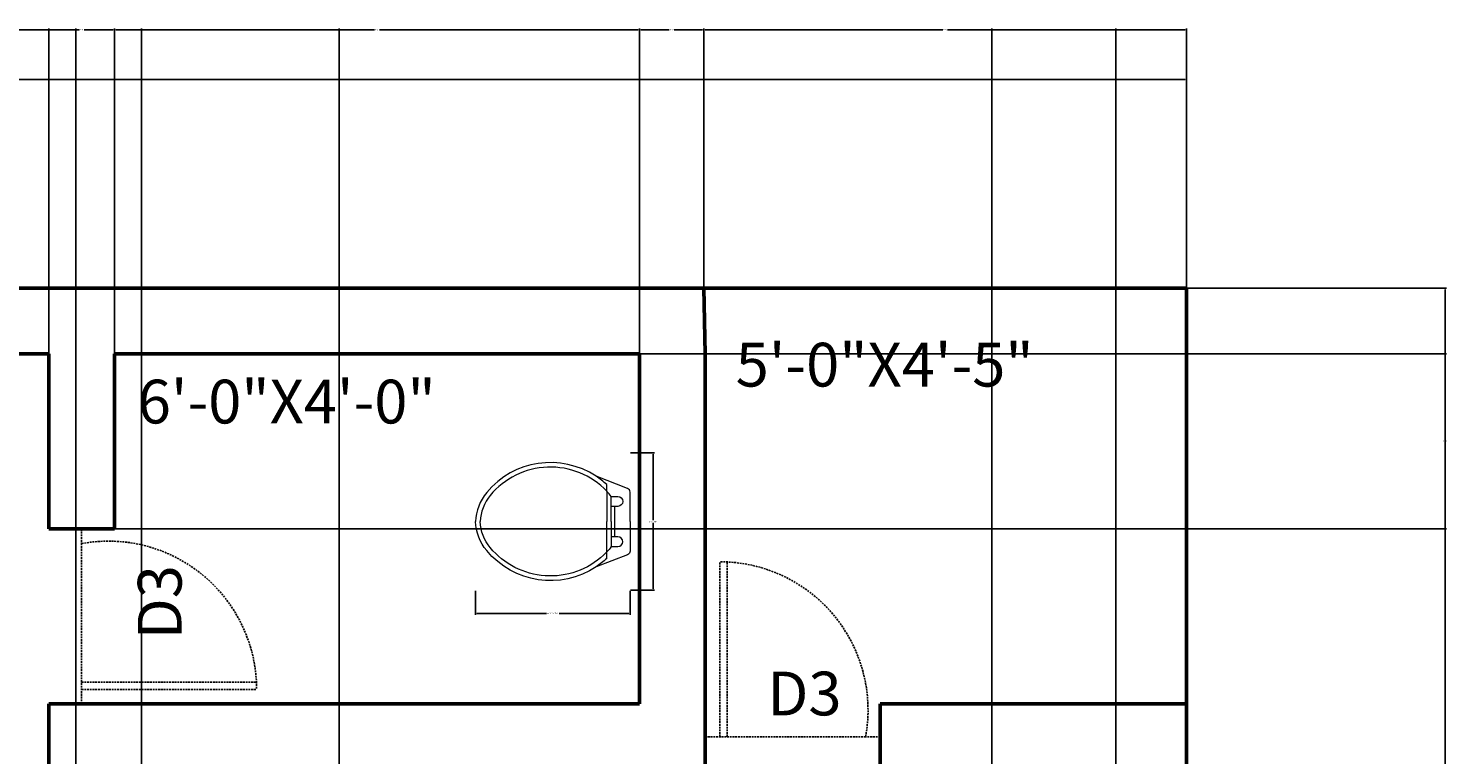
# Model space of a CAD drawing. Units: inches. Extents: x 3 to 576, y -689 to 51.
# Tile 21 of 21: x 381 to 576, y -48 to 51. Entities that reach past the tile are written whole.
import ezdxf

# ---------------------------------------------------------------- set-up
doc = ezdxf.new("R2010")
doc.units = ezdxf.units.IN
doc.header["$MEASUREMENT"] = 0
doc.linetypes.add('DASHED2', pattern=[0.375, 0.25, -0.125])
for name, color, linetype, lineweight in [('A-ANNO-DIMS', 2, 'Continuous', 18), ('A-ANNO-TEXT', 3, 'Continuous', 18), ('A-AREA-IDEN', 7, 'Continuous', 18), ('A-DOOR', 4, 'DASHED2', 25), ('A-FLOR-FIXT', 9, 'Continuous', 18), ('A-WALL', 7, 'Continuous', 50)]:
    doc.layers.add(name, color=color, linetype=linetype, lineweight=lineweight)
doc.styles.get("Standard").update_dxf_attribs({"font": 'arial.ttf'})
doc.dimstyles.get("Standard").update_dxf_attribs({"dimtxt": 0.18, "dimasz": 0.18, "dimexe": 0.18, "dimexo": 0.0625, "dimgap": 0.09, "dimtad": 0, "dimtih": 1, "dimtoh": 1, "dimdec": 0, "dimzin": 0, "dimdsep": 46, "dimlunit": 3, "dimtxsty": 'Standard', "dimcen": 0.09, "dimadec": 0, "dimazin": 0, "dimtfac": 1, "dimtdec": 0, "dimtofl": 0, "dimtmove": 0, "dimatfit": 3, "dimfxl": 1, "dimtolj": 1, "dimtzin": 0, "dimarcsym": 0})

# ---------------------------------------------------------------- blocks, each defined once
blk = doc.blocks.new('*D1')
at = {"layer": 'A-ANNO-DIMS', "color": 0, "lineweight": -2, "transparency": 16777216}
for p, q in [((38.29, 15.75), (38.29, 44.49)), ((38.47, 44.31), (276.45, 44.31)), ((540.11, 44.31), (302.14, 44.31)), ((540.29, 15.75), (540.29, 44.49))]:
    blk.add_line(p, q, dxfattribs=at)
at = {"layer": 'A-ANNO-DIMS', "color": 0, "transparency": 16777216}
for points in [[(38.47, 44.34), (38.47, 44.28), (38.29, 44.31)], [(540.11, 44.34), (540.11, 44.28), (540.29, 44.31)]]:
    blk.add_solid(points, dxfattribs=at)
at = {"layer": 'Defpoints', "color": 0, "transparency": 16777216}
for p in [(540.29, 44.31), (38.29, 15.69), (540.29, 15.69)]:
    blk.add_point(p, dxfattribs=at)
at = {"layer": 'A-ANNO-DIMS', "color": 0, "transparency": 16777216, "insert": (289.29, 44.31), "char_height": 6, "attachment_point": 5}
blk.add_mtext('\\A1;41\'-10"', dxfattribs=at)
blk = doc.blocks.new('WC-2')
for p, q in [((17.99, 12.27), (17.99, 13.16)), ((17.99, 12.27), (17.99, 8.1)), ((17.99, 3.93), (17.99, 8.1)), ((17.99, 3.04), (17.99, 3.93))]:
    blk.add_line(p, q)
for points in [[(16.53, 14.3, 0.383919), (1.53, 12.08, 0.163732), (0, 8.1, 0.359733)], [(17.99, 12.27, 0.448546), (2.02, 11.68, 0.162618), (0.63, 8.1, 0.470877)], [(17.99, 13.16, 0.040937), (16.53, 14.3, 0.163732)], [(21.19, 8.1), (21.19, 12.14, 0.31031), (20.85, 12.64), (16.53, 14.3, 0.209071)], [(18.62, 11.54, 0.022712), (17.99, 12.27, 0.162618)], [(18.62, 8.1), (18.62, 11.54, 0.476108)], [(18.62, 11.54), (19.51, 11.54, -1), (19.51, 10.18), (19.05, 10.18)], [(16.53, 1.89, -0.383919), (1.53, 4.11, -0.163732), (0, 8.1, -0.359733)], [(17.55, 3.5, -0.431639), (2.02, 4.52, -0.162618), (0.63, 8.1, -0.470877)], [(21.19, 8.1), (21.19, 4.05, -0.31031), (20.85, 3.55), (16.53, 1.89, -0.209071)], [(18.62, 8.1), (18.62, 4.66, -0.022712)], [(18.62, 4.66), (19.51, 4.66, 1), (19.51, 6.01), (19.05, 6.01)], [(17.99, 3.93, -0.014165), (17.55, 3.5, -0.162618)], [(18.62, 4.66, -0.022712), (17.99, 3.93, -0.162618)], [(17.99, 3.04, -0.040937), (16.53, 1.89, -0.163732)]]:
    blk.add_lwpolyline(points, format="xyb")
for points in [[(19.05, 10.18), (18.62, 10.18)], [(19.05, 10.18), (19.05, 6.01)], [(19.05, 6.01), (18.62, 6.01)]]:
    blk.add_lwpolyline(points)
blk = doc.blocks.new('DOOR-SWING-750')
for p, q in [((24, 24), (24, 22)), ((24, 22), (24, 2)), ((24, 2), (0, 2)), ((24, 0), (24, 2))]:
    blk.add_line(p, q)
blk.add_arc((20.33, 2), 20.33, 79.6111, 180)
blk = doc.blocks.new('*D37')
at = {"layer": 'A-ANNO-DIMS', "color": 0, "lineweight": -2, "transparency": 16777216}
for p, q in [((442.79, -25.78), (442.79, -29.08)), ((463.99, -25.78), (463.99, -29.08)), ((442.97, -28.9), (452.51, -28.9)), ((463.81, -28.9), (454.28, -28.9))]:
    blk.add_line(p, q, dxfattribs=at)
at = {"layer": 'A-ANNO-DIMS', "color": 0, "transparency": 16777216}
for points in [[(442.97, -28.87), (442.97, -28.93), (442.79, -28.9)], [(463.81, -28.87), (463.81, -28.93), (463.99, -28.9)]]:
    blk.add_solid(points, dxfattribs=at)
at = {"layer": 'Defpoints', "color": 0, "transparency": 16777216}
for p in [(442.79, -25.72), (463.99, -25.72), (463.99, -28.9)]:
    blk.add_point(p, dxfattribs=at)
at = {"layer": 'A-ANNO-DIMS', "color": 0, "transparency": 16777216, "insert": (453.39, -28.9), "char_height": 0.18, "attachment_point": 5}
blk.add_mtext('\\A1;WC 1\'-9" TYP.', dxfattribs=at)
blk = doc.blocks.new('*D38')
at = {"layer": 'A-ANNO-DIMS', "color": 0, "lineweight": -2, "transparency": 16777216}
for p, q in [((464.05, -6.89), (467.35, -6.89)), ((467.17, -7.07), (467.17, -16.12)), ((467.17, -25.54), (467.17, -16.49)), ((464.05, -25.72), (467.35, -25.72))]:
    blk.add_line(p, q, dxfattribs=at)
at = {"layer": 'A-ANNO-DIMS', "color": 0, "transparency": 16777216}
for points in [[(467.14, -7.07), (467.2, -7.07), (467.17, -6.89)], [(467.14, -25.54), (467.2, -25.54), (467.17, -25.72)]]:
    blk.add_solid(points, dxfattribs=at)
at = {"layer": 'Defpoints', "color": 0, "transparency": 16777216}
for p in [(463.99, -6.89), (467.17, -6.89), (463.99, -25.72)]:
    blk.add_point(p, dxfattribs=at)
at = {"layer": 'A-ANNO-DIMS', "color": 0, "transparency": 16777216, "insert": (467.17, -16.31), "char_height": 0.18, "attachment_point": 5}
blk.add_mtext('\\A1;1\'-7" TYP.', dxfattribs=at)
blk = doc.blocks.new('*D39')
at = {"layer": 'A-ANNO-DIMS', "color": 0, "lineweight": -2, "transparency": 16777216}
for p, q in [((540.36, 15.69), (575.92, 15.69)), ((575.74, 15.51), (575.74, -318.63)), ((575.74, -653.13), (575.74, -318.99)), ((540.36, -653.31), (575.92, -653.31))]:
    blk.add_line(p, q, dxfattribs=at)
at = {"layer": 'A-ANNO-DIMS', "color": 0, "transparency": 16777216}
for points in [[(575.71, 15.51), (575.77, 15.51), (575.74, 15.69)], [(575.71, -653.13), (575.77, -653.13), (575.74, -653.31)]]:
    blk.add_solid(points, dxfattribs=at)
at = {"layer": 'Defpoints', "color": 0, "transparency": 16777216}
for p in [(540.29, 15.69), (540.29, -653.31), (575.74, -653.31)]:
    blk.add_point(p, dxfattribs=at)
at = {"layer": 'A-ANNO-DIMS', "color": 0, "transparency": 16777216, "insert": (575.74, -318.81), "char_height": 0.18, "attachment_point": 5}
blk.add_mtext('\\A1;55\'-9"', dxfattribs=at)
blk = doc.blocks.new('*D44')
at = {"layer": 'A-ANNO-DIMS', "color": 0, "lineweight": -2, "transparency": 16777216}
for p, q in [((264.29, 6.75), (264.29, 51.32)), ((264.47, 51.14), (323.9, 51.14)), ((384.11, 51.14), (324.68, 51.14)), ((384.29, 6.75), (384.29, 51.32))]:
    blk.add_line(p, q, dxfattribs=at)
at = {"layer": 'A-ANNO-DIMS', "color": 0, "transparency": 16777216}
for points in [[(264.47, 51.17), (264.47, 51.11), (264.29, 51.14)], [(384.11, 51.17), (384.11, 51.11), (384.29, 51.14)]]:
    blk.add_solid(points, dxfattribs=at)
at = {"layer": 'Defpoints', "color": 0, "transparency": 16777216}
for p in [(384.29, 51.14), (264.29, 6.69), (384.29, 6.69)]:
    blk.add_point(p, dxfattribs=at)
at = {"layer": 'A-ANNO-DIMS', "color": 0, "transparency": 16777216, "insert": (324.29, 51.14), "char_height": 0.18, "attachment_point": 5}
blk.add_mtext('\\A1;10\'-0"', dxfattribs=at)
blk = doc.blocks.new('*D45')
at = {"layer": 'A-ANNO-DIMS', "color": 0, "lineweight": -2, "transparency": 16777216}
for p, q in [((384.29, 6.75), (384.29, 51.32)), ((384.47, 51.14), (388.46, 51.14)), ((393.11, 51.14), (389.12, 51.14)), ((393.29, 6.75), (393.29, 51.32))]:
    blk.add_line(p, q, dxfattribs=at)
at = {"layer": 'A-ANNO-DIMS', "color": 0, "transparency": 16777216}
for points in [[(384.47, 51.17), (384.47, 51.11), (384.29, 51.14)], [(393.11, 51.17), (393.11, 51.11), (393.29, 51.14)]]:
    blk.add_solid(points, dxfattribs=at)
at = {"layer": 'Defpoints', "color": 0, "transparency": 16777216}
for p in [(393.29, 51.14), (384.29, 6.69), (393.29, 6.69)]:
    blk.add_point(p, dxfattribs=at)
at = {"layer": 'A-ANNO-DIMS', "color": 0, "transparency": 16777216, "insert": (388.79, 51.14), "char_height": 0.18, "attachment_point": 5}
blk.add_mtext('\\A1;0\'-9"', dxfattribs=at)
blk = doc.blocks.new('*D46')
at = {"layer": 'A-ANNO-DIMS', "color": 0, "lineweight": -2, "transparency": 16777216}
for p, q in [((393.29, 6.75), (393.29, 51.32)), ((393.47, 51.14), (428.96, 51.14)), ((465.11, 51.14), (429.62, 51.14)), ((465.29, 6.75), (465.29, 51.32))]:
    blk.add_line(p, q, dxfattribs=at)
at = {"layer": 'A-ANNO-DIMS', "color": 0, "transparency": 16777216}
for points in [[(393.47, 51.17), (393.47, 51.11), (393.29, 51.14)], [(465.11, 51.17), (465.11, 51.11), (465.29, 51.14)]]:
    blk.add_solid(points, dxfattribs=at)
at = {"layer": 'Defpoints', "color": 0, "transparency": 16777216}
for p in [(465.29, 51.14), (393.29, 6.69), (465.29, 6.69)]:
    blk.add_point(p, dxfattribs=at)
at = {"layer": 'A-ANNO-DIMS', "color": 0, "transparency": 16777216, "insert": (429.29, 51.14), "char_height": 0.18, "attachment_point": 5}
blk.add_mtext('\\A1;6\'-0"', dxfattribs=at)
blk = doc.blocks.new('*D47')
at = {"layer": 'A-ANNO-DIMS', "color": 0, "lineweight": -2, "transparency": 16777216}
for p, q in [((465.29, 6.75), (465.29, 51.32)), ((465.47, 51.14), (469.37, 51.14)), ((473.93, 51.14), (470.03, 51.14)), ((474.11, 15.75), (474.11, 51.32))]:
    blk.add_line(p, q, dxfattribs=at)
at = {"layer": 'A-ANNO-DIMS', "color": 0, "transparency": 16777216}
for points in [[(465.47, 51.17), (465.47, 51.11), (465.29, 51.14)], [(473.93, 51.17), (473.93, 51.11), (474.11, 51.14)]]:
    blk.add_solid(points, dxfattribs=at)
at = {"layer": 'Defpoints', "color": 0, "transparency": 16777216}
for p in [(474.11, 51.14), (474.11, 15.69), (465.29, 6.69)]:
    blk.add_point(p, dxfattribs=at)
at = {"layer": 'A-ANNO-DIMS', "color": 0, "transparency": 16777216, "insert": (469.7, 51.14), "char_height": 0.18, "attachment_point": 5}
blk.add_mtext('\\A1;0\'-9"', dxfattribs=at)
blk = doc.blocks.new('*D48')
at = {"layer": 'A-ANNO-DIMS', "color": 0, "lineweight": -2, "transparency": 16777216}
for p, q in [((474.11, 15.75), (474.11, 51.32)), ((474.29, 51.14), (506.87, 51.14)), ((540.11, 51.14), (507.53, 51.14)), ((540.29, 15.75), (540.29, 51.32))]:
    blk.add_line(p, q, dxfattribs=at)
at = {"layer": 'A-ANNO-DIMS', "color": 0, "transparency": 16777216}
for points in [[(474.29, 51.17), (474.29, 51.11), (474.11, 51.14)], [(540.11, 51.17), (540.11, 51.11), (540.29, 51.14)]]:
    blk.add_solid(points, dxfattribs=at)
at = {"layer": 'Defpoints', "color": 0, "transparency": 16777216}
for p in [(540.29, 51.14), (474.11, 15.69), (540.29, 15.69)]:
    blk.add_point(p, dxfattribs=at)
at = {"layer": 'A-ANNO-DIMS', "color": 0, "transparency": 16777216, "insert": (507.2, 51.14), "char_height": 0.18, "attachment_point": 5}
blk.add_mtext('\\A1;5\'-6"', dxfattribs=at)
blk = doc.blocks.new('*D64')
at = {"layer": 'A-ANNO-DIMS', "color": 0, "lineweight": -2, "transparency": 16777216}
for p, q in [((540.23, 15.69), (2.66, 15.69)), ((2.84, 15.51), (2.84, -17.13)), ((2.84, -50.13), (2.84, -17.49)), ((531.23, -50.31), (2.66, -50.31))]:
    blk.add_line(p, q, dxfattribs=at)
at = {"layer": 'A-ANNO-DIMS', "color": 0, "transparency": 16777216}
for points in [[(2.81, 15.51), (2.87, 15.51), (2.84, 15.69)], [(2.81, -50.13), (2.87, -50.13), (2.84, -50.31)]]:
    blk.add_solid(points, dxfattribs=at)
at = {"layer": 'Defpoints', "color": 0, "transparency": 16777216}
for p in [(540.29, 15.69), (2.84, -50.31), (531.29, -50.31)]:
    blk.add_point(p, dxfattribs=at)
at = {"layer": 'A-ANNO-DIMS', "color": 0, "transparency": 16777216, "insert": (2.84, -17.31), "char_height": 0.18, "attachment_point": 5}
blk.add_mtext('\\A1;5\'-6"', dxfattribs=at)
blk = doc.blocks.new('*D96')
at = {"layer": 'A-ANNO-DIMS', "color": 0, "lineweight": -2, "transparency": 16777216}
for p, q in [((397.02, -506.04), (397.02, 51.32)), ((397.2, 51.14), (410.22, 51.14)), ((423.91, 51.14), (410.89, 51.14)), ((424.09, -506.04), (424.09, 51.32))]:
    blk.add_line(p, q, dxfattribs=at)
at = {"layer": 'A-ANNO-DIMS', "color": 0, "transparency": 16777216}
for points in [[(397.2, 51.17), (397.2, 51.11), (397.02, 51.14)], [(423.91, 51.17), (423.91, 51.11), (424.09, 51.14)]]:
    blk.add_solid(points, dxfattribs=at)
at = {"layer": 'Defpoints', "color": 0, "transparency": 16777216}
for p in [(424.09, 51.14), (397.02, -506.1), (424.09, -506.1)]:
    blk.add_point(p, dxfattribs=at)
at = {"layer": 'A-ANNO-DIMS', "color": 0, "transparency": 16777216, "insert": (410.56, 51.14), "char_height": 0.18, "attachment_point": 5}
blk.add_mtext('\\A1;2\'-3"', dxfattribs=at)
blk = doc.blocks.new('*D102')
at = {"layer": 'A-ANNO-DIMS', "color": 0, "lineweight": -2, "transparency": 16777216}
for p, q in [((393.36, 6.69), (575.92, 6.69)), ((575.74, 6.51), (575.74, -5.13)), ((575.74, -17.13), (575.74, -5.49)), ((393.36, -17.31), (575.92, -17.31))]:
    blk.add_line(p, q, dxfattribs=at)
at = {"layer": 'A-ANNO-DIMS', "color": 0, "transparency": 16777216}
for points in [[(575.71, 6.51), (575.77, 6.51), (575.74, 6.69)], [(575.71, -17.13), (575.77, -17.13), (575.74, -17.31)]]:
    blk.add_solid(points, dxfattribs=at)
at = {"layer": 'Defpoints', "color": 0, "transparency": 16777216}
for p in [(393.29, 6.69), (393.29, -17.31), (575.74, -17.31)]:
    blk.add_point(p, dxfattribs=at)
at = {"layer": 'A-ANNO-DIMS', "color": 0, "transparency": 16777216, "insert": (575.74, -5.31), "char_height": 0.18, "attachment_point": 5}
blk.add_mtext('\\A1;2\'-0"', dxfattribs=at)
blk = doc.blocks.new('*D118')
at = {"layer": 'A-ANNO-DIMS', "color": 0, "lineweight": -2, "transparency": 16777216}
for p, q in [((352.02, -506.25), (352.02, 51.32)), ((352.2, 51.14), (369.69, 51.14)), ((387.84, 51.14), (370.35, 51.14)), ((388.02, -506.25), (388.02, 51.32))]:
    blk.add_line(p, q, dxfattribs=at)
at = {"layer": 'A-ANNO-DIMS', "color": 0, "transparency": 16777216}
for points in [[(352.2, 51.17), (352.2, 51.11), (352.02, 51.14)], [(387.84, 51.17), (387.84, 51.11), (388.02, 51.14)]]:
    blk.add_solid(points, dxfattribs=at)
at = {"layer": 'Defpoints', "color": 0, "transparency": 16777216}
for p in [(388.02, 51.14), (352.02, -506.31), (388.02, -506.31)]:
    blk.add_point(p, dxfattribs=at)
at = {"layer": 'A-ANNO-DIMS', "color": 0, "transparency": 16777216, "insert": (370.02, 51.14), "char_height": 0.18, "attachment_point": 5}
blk.add_mtext('\\A1;3\'-0"', dxfattribs=at)
blk = doc.blocks.new('*D124')
at = {"layer": 'A-ANNO-DIMS', "color": 0, "lineweight": -2, "transparency": 16777216}
for p, q in [((513.61, -235.44), (513.61, 51.32)), ((513.79, 51.14), (521.77, 51.14)), ((530.39, 51.14), (522.41, 51.14)), ((530.57, -227.22), (530.57, 51.32))]:
    blk.add_line(p, q, dxfattribs=at)
at = {"layer": 'A-ANNO-DIMS', "color": 0, "transparency": 16777216}
for points in [[(513.79, 51.17), (513.79, 51.11), (513.61, 51.14)], [(530.39, 51.17), (530.39, 51.11), (530.57, 51.14)]]:
    blk.add_solid(points, dxfattribs=at)
at = {"layer": 'Defpoints', "color": 0, "transparency": 16777216}
for p in [(530.57, 51.14), (530.57, -227.28), (513.61, -235.5)]:
    blk.add_point(p, dxfattribs=at)
at = {"layer": 'A-ANNO-DIMS', "color": 0, "transparency": 16777216, "insert": (522.09, 51.14), "char_height": 0.18, "attachment_point": 5}
blk.add_mtext('\\A1;1\'-5"', dxfattribs=at)

msp = doc.modelspace()

# ---------------------------------------------------------------- linework, layer by layer
at = {"layer": 'A-DOOR'}
for p, q in [((477.29, -45.81), (477.29, -21.81)), ((388.79, -38.31), (412.79, -38.31))]:
    msp.add_line(p, q, dxfattribs=at)
at = {"layer": 'A-WALL'}
for p, q in [((38.29, 15.69), (540.29, 15.69)), ((474.11, 15.69), (474.29, 6.69)), ((540.29, 15.69), (540.29, -653.31)), ((264.29, 6.69), (384.29, 6.69)), ((384.29, 6.69), (384.29, -17.31)), ((393.29, 6.69), (393.29, -17.31)), ((393.29, 6.69), (465.29, 6.69)), ((465.29, 6.69), (465.29, -41.31)), ((474.29, 6.69), (474.29, -50.31)), ((393.29, -17.31), (384.29, -17.31)), ((393.29, -41.31), (384.29, -41.31)), ((384.29, -41.31), (384.29, -125.31)), ((393.29, -41.31), (465.29, -41.31)), ((498.29, -41.31), (498.29, -50.31)), ((498.29, -41.31), (540.29, -41.31))]:
    msp.add_line(p, q, dxfattribs=at)

# ---------------------------------------------------------------- block references
at = {"layer": 'A-DOOR', "extrusion": (0, 0, -1), "zscale": -1}
msp.add_blockref('DOOR-SWING-750', (-412.79, -41.31), dxfattribs=at)
at = {"layer": 'A-DOOR', "rotation": 269.9999999999999}
msp.add_blockref('DOOR-SWING-750', (474.29, -21.81), dxfattribs=at)
at = {"layer": 'A-FLOR-FIXT'}
msp.add_blockref('WC-2', (442.8, -24.4), dxfattribs=at)

# ---------------------------------------------------------------- texts
at = {"layer": 'A-ANNO-TEXT', "insert": (396.5, -32.45), "char_height": 6, "attachment_point": 1, "rotation": 90}
msp.add_mtext('D3', dxfattribs=at)
at = {"layer": 'A-ANNO-TEXT', "insert": (482.81, -36.88), "char_height": 6, "attachment_point": 1}
msp.add_mtext('D3', dxfattribs=at)
at = {"layer": 'A-AREA-IDEN', "insert": (478.47, 8.21), "char_height": 6, "attachment_point": 1}
msp.add_mtext_dynamic_manual_height_columns('5\'-0"X4\'-5"', width=0.2177, gutter_width=1, heights=[0], dxfattribs=at)
at = {"layer": 'A-AREA-IDEN', "insert": (396.49, 3.15), "char_height": 6, "attachment_point": 1}
msp.add_mtext('6\'-0"X4\'-0"', dxfattribs=at)

# ---------------------------------------------------------------- dimensions: what is measured, and where the dimension line sits
at = {"layer": 'A-ANNO-DIMS'}
for base, p1, p2, override, picture, middle in [((384.29, 51.14), (264.29, 6.69), (384.29, 6.69), {"dimdec": 1, "dimlfac": 1, "dimrnd": 0, "dimzin": 1, "dimdsep": 46, "dimlunit": 4, "dimfrac": 2}, '*D44', (324.29, 51.14)), ((388.02, 51.14), (352.02, -506.31), (388.02, -506.31), {"dimdec": 1, "dimlfac": 1, "dimrnd": 0, "dimzin": 1, "dimdsep": 46, "dimlunit": 4, "dimfrac": 2}, '*D118', (370.02, 51.14)), ((393.29, 51.14), (384.29, 6.69), (393.29, 6.69), {"dimdec": 1, "dimlfac": 1, "dimrnd": 0, "dimzin": 1, "dimdsep": 46, "dimlunit": 4, "dimfrac": 2}, '*D45', (388.79, 51.14)), ((465.29, 51.14), (393.29, 6.69), (465.29, 6.69), {"dimdec": 1, "dimlfac": 1, "dimrnd": 0, "dimzin": 1, "dimdsep": 46, "dimlunit": 4, "dimfrac": 2}, '*D46', (429.29, 51.14)), ((424.09, 51.14), (397.02, -506.1), (424.09, -506.1), {"dimdec": 1, "dimlfac": 1, "dimrnd": 0, "dimzin": 1, "dimdsep": 46, "dimlunit": 4, "dimfrac": 2}, '*D96', (410.56, 51.14)), ((474.11, 51.14), (465.29, 6.69), (474.11, 15.69), {"dimdec": 1, "dimlfac": 1, "dimrnd": 0, "dimzin": 1, "dimdsep": 46, "dimlunit": 4, "dimfrac": 2}, '*D47', (469.7, 51.14)), ((540.29, 51.14), (474.11, 15.69), (540.29, 15.69), {"dimdec": 1, "dimlfac": 1, "dimrnd": 0, "dimzin": 1, "dimdsep": 46, "dimlunit": 4, "dimfrac": 2}, '*D48', (507.2, 51.14)), ((530.57, 51.14), (513.61, -235.5), (530.57, -227.28), {"dimdec": 1, "dimlfac": 1, "dimrnd": 0, "dimzin": 1, "dimdsep": 46, "dimlunit": 4, "dimfrac": 2}, '*D124', (522.09, 51.14)), ((540.29, 44.31), (38.29, 15.69), (540.29, 15.69), {"dimtxt": 6, "dimclrd": 0, "dimclre": 0, "dimclrt": 0}, '*D1', (289.29, 44.31))]:
    dim = msp.add_linear_dim(base=base, p1=p1, p2=p2, dimstyle='Standard', override=override, dxfattribs=at)
    dim.commit()
    dim.dimension.update_dxf_attribs({"geometry": picture, "text_midpoint": middle})
for base, p1, p2, picture, middle in [((2.84, -50.31), (540.29, 15.69), (531.29, -50.31), '*D64', (2.84, -17.31)), ((575.74, -653.31), (540.29, 15.69), (540.29, -653.31), '*D39', (575.74, -318.81)), ((575.74, -17.31), (393.29, 6.69), (393.29, -17.31), '*D102', (575.74, -5.31))]:
    dim = msp.add_linear_dim(base=base, p1=p1, p2=p2, angle=90, dimstyle='Standard', override={"dimdec": 1, "dimlfac": 1, "dimrnd": 0, "dimzin": 1, "dimdsep": 46, "dimlunit": 4, "dimfrac": 2}, dxfattribs=at)
    dim.commit()
    dim.dimension.update_dxf_attribs({"geometry": picture, "text_midpoint": middle})
dim = msp.add_linear_dim(base=(467.17, -6.89), p1=(463.99, -25.72), p2=(463.99, -6.89), angle=90, text='<> TYP.', dimstyle='Standard', override={"dimdec": 1, "dimlfac": 1, "dimrnd": 0, "dimzin": 1, "dimdsep": 46, "dimlunit": 4, "dimfrac": 2}, dxfattribs=at)
dim.commit()
dim.dimension.update_dxf_attribs({"geometry": '*D38', "text_midpoint": (467.17, -16.31)})
dim = msp.add_linear_dim(base=(463.99, -28.9), p1=(442.79, -25.72), p2=(463.99, -25.72), text='WC <> TYP.', dimstyle='Standard', override={"dimdec": 1, "dimlfac": 1, "dimrnd": 0, "dimzin": 1, "dimdsep": 46, "dimlunit": 4, "dimfrac": 2}, dxfattribs=at)
dim.commit()
dim.dimension.update_dxf_attribs({"geometry": '*D37', "text_midpoint": (453.39, -28.9)})

doc.saveas('drawing.dxf')
